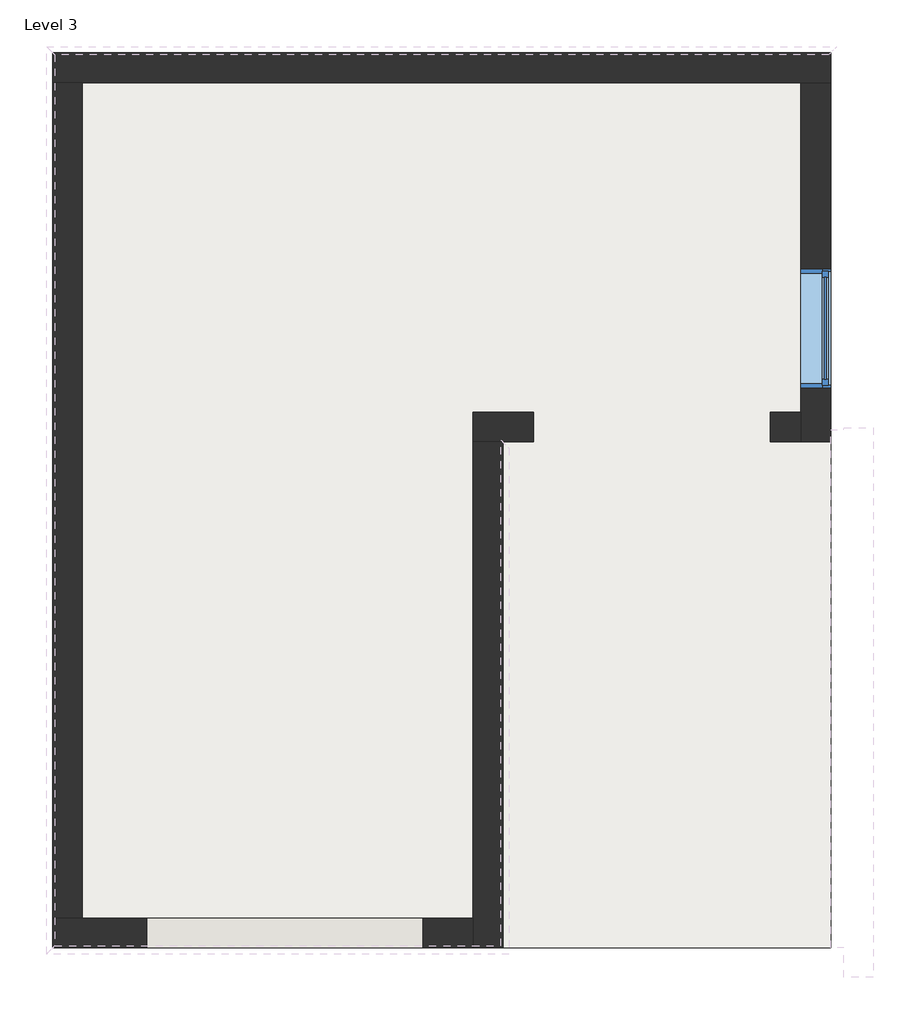
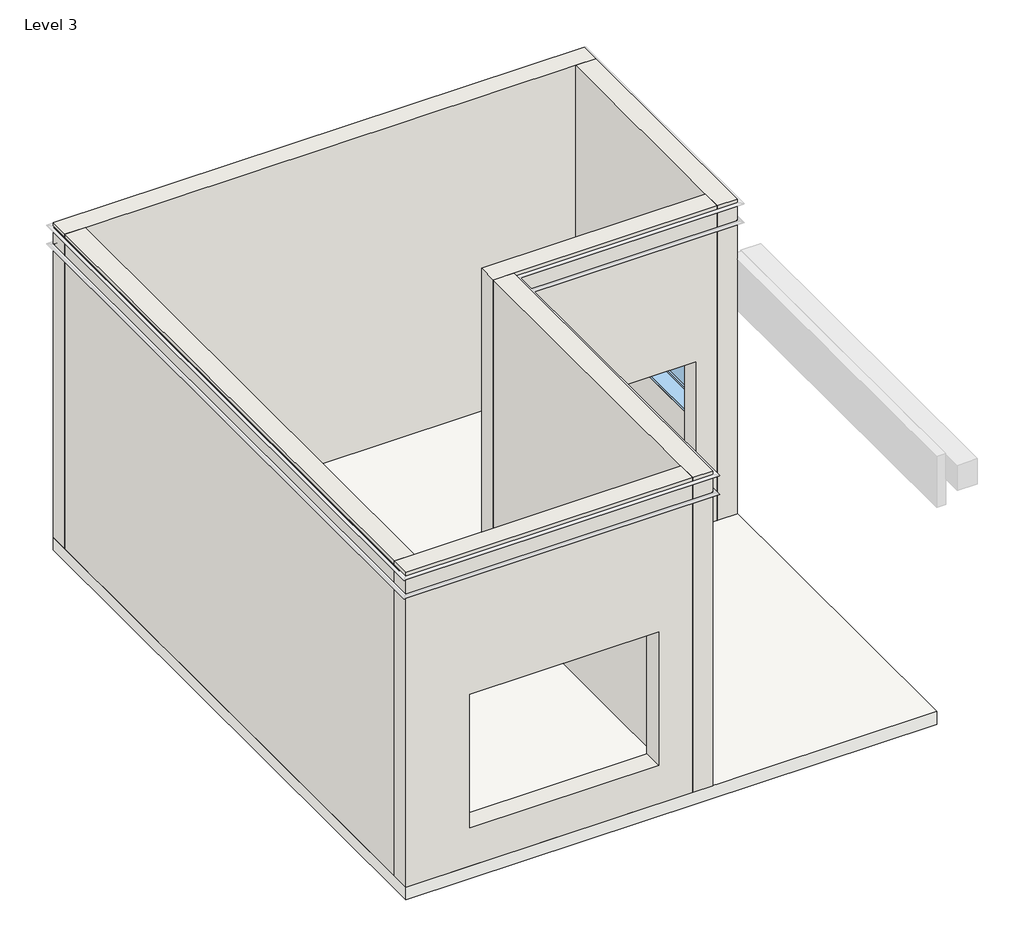
# One storey, part 1 of 2: 6 walls, 1 slab, 1 window.
"""IFC4 building model written with IfcOpenShell, lengths in millimetres."""

from ifc_helpers import new_model, si_unit, point, frame, frame_2d, origin, place, context, project, spatial, polyline, circle_curve, ellipse_curve, trimmed, segment, composite_curve, outline, extrude, faceted_brep, transform, mapped, element, save
from ifc_brep_helpers import plane_surface, cylinder_surface, advanced_brep
from components import window_c1f32544

model = new_model("IFC4")

# Units and contexts
model_context = context("Model", 3, world=origin())
ifc_project = project(units=[si_unit("LENGTHUNIT", "METRE", prefix="MILLI")], contexts=[model_context])

# Site, building, storey
site = spatial("IfcSite", under=ifc_project)
building = spatial("IfcBuilding", under=site)
storey = spatial("IfcBuildingStorey", under=building, Name="Level 3", Elevation=3200.4)

# Slab
placement = place(None, origin())
element("IfcSlab", 1, ObjectType="6\" floor", at=placement, inside=storey, context=model_context, shape_type="SweptSolid", body=[
    extrude(outline(polyline([(-7274.9953834, 7640.1262137), (-7274.9953834, 740.1262137), (-13274.9953834, 740.1262137), (-13274.9953834, 7640.1262137), (-7274.9953834, 7640.1262137)])), frame((0.0, 0.0, 3048.0), z_axis=(0.0, 0.0, 1.0), x_axis=(1.0, 0.0, 0.0)), (0.0, 0.0, 1.0), 152.4),
])

# Walls
element("IfcWall", 2, ObjectType="9\" wall", at=placement, inside=storey, context=model_context, shape_type="SolidModel", body=[
    faceted_brep([(-13274.9953834, 7411.5262137, 3200.4), (-13046.3953834, 7411.5262137, 3200.4), (-7503.5953834, 7411.5262137, 3200.4), (-7274.9953834, 7411.5262137, 3200.4), (-7274.9953834, 7411.5262137, 6692.9), (-7289.8797834, 7411.5262137, 6692.9), (-7289.8797834, 7411.5262137, 6921.5), (-7274.9953834, 7411.5262137, 6921.5), (-7274.9953834, 7411.5262137, 6962.2619583), (-7503.5953834, 7411.5262137, 6962.2619583), (-13046.3953834, 7411.5262137, 6962.2619583), (-13274.9953834, 7411.5262137, 6962.2619583), (-13274.9953834, 7411.5262137, 6921.5), (-13260.1109834, 7411.5262137, 6921.5), (-13260.1109834, 7411.5262137, 6692.9), (-13274.9953834, 7411.5262137, 6692.9), (-7274.9953834, 7640.1262137, 3200.4), (-13274.9953834, 7640.1262137, 3200.4), (-13274.9953834, 7640.1262137, 6692.9), (-7274.9953834, 7640.1262137, 6692.9), (-13274.9953834, 7640.1262137, 6962.2619583), (-7274.9953834, 7640.1262137, 6962.2619583), (-7274.9953834, 7640.1262137, 6921.5), (-13274.9953834, 7640.1262137, 6921.5), (-7289.8797834, 7625.2418137, 6921.5), (-13260.1109834, 7625.2418137, 6921.5), (-13260.1109834, 7625.2418137, 6692.9), (-7289.8797834, 7625.2418137, 6692.9)], [[[0, 1, 2, 3, 4, 5, 6, 7, 8, 9, 10, 11, 12, 13, 14, 15]], [[16, 17, 18, 19]], [[20, 21, 22, 23]], [[3, 2, 1, 0, 17, 16]], [[11, 10, 9, 8, 21, 20]], [[3, 16, 19, 4]], [[21, 8, 7, 22]], [[11, 20, 23, 12]], [[17, 0, 15, 18]], [[24, 25, 13, 12, 23, 22, 7, 6]], [[26, 27, 5, 4, 19, 18, 15, 14]], [[25, 26, 14, 13]], [[25, 24, 27, 26]], [[27, 24, 6, 5]]]),
    advanced_brep(
    [(-13274.9953834, 7411.5262137, 6907.55311), (-13274.9953834, 7411.5262137, 6706.84689), (-13267.3499834, 7411.5262137, 6716.943989), (-13267.3499834, 7411.5262137, 6897.456011), (-7274.9953834, 7411.5262137, 6706.84689), (-7274.9953834, 7411.5262137, 6907.55311), (-7282.6407834, 7411.5262137, 6897.456011), (-7282.6407834, 7411.5262137, 6716.943989), (-13274.9953834, 7640.1262137, 6706.84689), (-13274.9953834, 7640.1262137, 6907.55311), (-7274.9953834, 7640.1262137, 6907.55311), (-7274.9953834, 7640.1262137, 6706.84689), (-13267.3499834, 7632.4808137, 6897.456011), (-13267.3499834, 7632.4808137, 6716.943989), (-7282.6407834, 7632.4808137, 6897.456011), (-7282.6407834, 7632.4808137, 6716.943989)],
    [
        (0, 1),
        (1, 2, circle_curve(frame((-13277.8401834, 7411.5262137, 6716.943989), z_axis=(0.0, -1.0, 0.0), x_axis=(-1.0, 0.0, 0.0)), 10.4902)),
        (2, 3),
        (3, 0, circle_curve(frame((-13277.8401834, 7411.5262137, 6897.456011), z_axis=(0.0, -1.0, 0.0), x_axis=(-1.0, 0.0, 0.0)), 10.4902)),
        (4, 5),
        (5, 6, circle_curve(frame((-7272.1505834, 7411.5262137, 6897.456011), z_axis=(0.0, -1.0, 0.0), x_axis=(1.0, 0.0, 0.0)), 10.4902)),
        (6, 7),
        (7, 4, circle_curve(frame((-7272.1505834, 7411.5262137, 6716.943989), z_axis=(0.0, -1.0, 0.0), x_axis=(1.0, 0.0, 0.0)), 10.4902)),
        (8, 9),
        (9, 10),
        (10, 11),
        (11, 8),
        (4, 11),
        (10, 5),
        (0, 9),
        (8, 1),
        (12, 9, ellipse_curve(frame((-13277.8401834, 7642.9710137, 6897.456011), z_axis=(-0.7071067811865492, -0.7071067811865458, 0.0), x_axis=(-0.7071067811865457, 0.7071067811865492, 0.0)), 14.8353831, 10.4902)),
        (3, 12),
        (13, 12),
        (2, 13),
        (8, 13, ellipse_curve(frame((-13277.8401834, 7642.9710137, 6716.943989), z_axis=(-0.7071067811865492, -0.7071067811865458, 0.0), x_axis=(-0.7071067811865457, 0.7071067811865492, 0.0)), 14.8353831, 10.4902)),
        (12, 14),
        (14, 10, ellipse_curve(frame((-7272.1505834, 7642.9710137, 6897.456011), z_axis=(-0.7071067811865445, 0.7071067811865505, 0.0), x_axis=(0.7071067811865507, 0.7071067811865445, 0.0)), 14.8353831, 10.4902)),
        (13, 15),
        (15, 14),
        (11, 15, ellipse_curve(frame((-7272.1505834, 7642.9710137, 6716.943989), z_axis=(-0.7071067811865445, 0.7071067811865505, 0.0), x_axis=(0.7071067811865507, 0.7071067811865445, 0.0)), 14.8353831, 10.4902)),
        (14, 6),
        (15, 7),
    ],
    [
        plane_surface(frame((-13274.9953834, 7411.5262137, 3200.4), z_axis=(0.0, -1.0, 0.0), x_axis=(1.0, 0.0, 0.0))),
        plane_surface(frame((-13274.9953834, 7640.1262137, 3200.4), z_axis=(0.0, 1.0, 0.0), x_axis=(-1.0, 0.0, 0.0))),
        plane_surface(frame((-7274.9953834, 7640.1262137, 3200.4), z_axis=(1.0, 0.0, 0.0), x_axis=(0.0, 1.0, 0.0))),
        plane_surface(frame((-13274.9953834, 740.1262137, 3200.4), z_axis=(-1.0, 0.0, 0.0), x_axis=(0.0, -1.0, 0.0))),
        cylinder_surface(frame((-13277.8401834, 740.1262137, 6897.456011), z_axis=(0.0, 1.0, 0.0), x_axis=(-1.0, 0.0, 0.0)), 10.4902),
        plane_surface(frame((-13267.3499834, 740.1262137, 6897.456011), z_axis=(1.0, 0.0, 0.0), x_axis=(0.0, 1.0, 0.0))),
        cylinder_surface(frame((-13277.8401834, 740.1262137, 6716.943989), z_axis=(0.0, 1.0, 0.0), x_axis=(-1.0, 0.0, 0.0)), 10.4902),
        cylinder_surface(frame((-13274.9953834, 7642.9710137, 6897.456011), z_axis=(1.0, 0.0, 0.0), x_axis=(0.0, 1.0, 0.0)), 10.4902),
        plane_surface(frame((-13267.3499834, 7632.4808137, 6897.456011), z_axis=(0.0, -1.0, 0.0), x_axis=(1.0, 0.0, 0.0))),
        cylinder_surface(frame((-13274.9953834, 7642.9710137, 6716.943989), z_axis=(1.0, 0.0, 0.0), x_axis=(0.0, 1.0, 0.0)), 10.4902),
        cylinder_surface(frame((-7272.1505834, 7640.1262137, 6897.456011), z_axis=(0.0, -1.0, 0.0), x_axis=(1.0, 0.0, 0.0)), 10.4902),
        plane_surface(frame((-7282.6407834, 7632.4808137, 6897.456011), z_axis=(-1.0, 0.0, 0.0), x_axis=(0.0, -1.0, 0.0))),
        cylinder_surface(frame((-7272.1505834, 7640.1262137, 6716.943989), z_axis=(0.0, -1.0, 0.0), x_axis=(1.0, 0.0, 0.0)), 10.4902),
    ],
    [
        (0, [[1, 2, 3, 4]]),
        (0, [[5, 6, 7, 8]]),
        (1, [[9, 10, 11, 12]]),
        (2, [[-5, 13, -11, 14]]),
        (3, [[-1, 15, -9, 16]]),
        (4, [[17, -15, -4, 18]]),
        (5, [[19, -18, -3, 20]]),
        (6, [[21, -20, -2, -16]]),
        (7, [[22, 23, -10, -17]]),
        (8, [[-19, 24, 25, -22]]),
        (9, [[-24, -21, -12, 26]]),
        (10, [[-23, 27, -6, -14]]),
        (11, [[-25, 28, -7, -27]]),
        (12, [[-26, -13, -8, -28]]),
    ],
),
])
element("IfcWall", 3, ObjectType="9\" wall", at=placement, inside=storey, context=model_context, shape_type="SolidModel", body=[
    faceted_brep([(-7503.5953834, 7411.5262137, 3200.4), (-7503.5953834, 4868.7176199, 3200.4), (-7503.5953834, 4640.1176199, 3200.4), (-7503.5953834, 4640.1176199, 6692.9), (-7503.5953834, 4655.0020199, 6692.9), (-7503.5953834, 4655.0020199, 6921.5), (-7503.5953834, 4640.1176199, 6921.5), (-7503.5953834, 4640.1176199, 6962.2619583), (-7503.5953834, 4868.7176199, 6962.2619583), (-7503.5953834, 7411.5262137, 6962.2619583), (-7503.5953834, 5059.2176199, 5334.0), (-7503.5953834, 5059.2176199, 4114.8), (-7503.5953834, 5973.6176199, 4114.8), (-7503.5953834, 5973.6176199, 5334.0), (-7274.9953834, 4640.1176199, 3200.4), (-7274.9953834, 7411.5262137, 3200.4), (-7274.9953834, 7411.5262137, 6692.9), (-7274.9953834, 4640.1176199, 6692.9), (-7274.9953834, 5059.2176199, 4114.8), (-7274.9953834, 5059.2176199, 5334.0), (-7274.9953834, 5973.6176199, 5334.0), (-7274.9953834, 5973.6176199, 4114.8), (-7274.9953834, 7411.5262137, 6962.2619583), (-7274.9953834, 4640.1176199, 6962.2619583), (-7274.9953834, 4640.1176199, 6921.5), (-7274.9953834, 7411.5262137, 6921.5), (-7289.8797834, 7411.5262137, 6921.5), (-7289.8797834, 7411.5262137, 6692.9), (-7289.8797834, 4655.0020199, 6921.5), (-7289.8797834, 4655.0020199, 6692.9)], [[[0, 1, 2, 3, 4, 5, 6, 7, 8, 9], [10, 11, 12, 13]], [[14, 15, 16, 17], [18, 19, 20, 21]], [[22, 23, 24, 25]], [[2, 1, 0, 15, 14]], [[9, 8, 7, 23, 22]], [[0, 9, 22, 25, 26, 27, 16, 15]], [[11, 10, 19, 18]], [[12, 11, 18, 21]], [[13, 12, 21, 20]], [[10, 13, 20, 19]], [[2, 14, 17, 3]], [[23, 7, 6, 24]], [[5, 28, 26, 25, 24, 6]], [[27, 29, 4, 3, 17, 16]], [[28, 29, 27, 26]], [[29, 28, 5, 4]]]),
    advanced_brep(
    [(-7503.5953834, 4640.1176199, 6706.84689), (-7503.5953834, 4640.1176199, 6907.55311), (-7503.5953834, 4647.7630199, 6897.456011), (-7503.5953834, 4647.7630199, 6716.943989), (-7274.9953834, 7411.5262137, 6706.84689), (-7274.9953834, 7411.5262137, 6907.55311), (-7274.9953834, 4640.1176199, 6907.55311), (-7274.9953834, 4640.1176199, 6706.84689), (-7282.6407834, 7411.5262137, 6716.943989), (-7282.6407834, 7411.5262137, 6897.456011), (-7282.6407834, 4647.7630199, 6897.456011), (-7282.6407834, 4647.7630199, 6716.943989)],
    [
        (0, 1),
        (1, 2, circle_curve(frame((-7503.5953834, 4637.2728199, 6897.456011), z_axis=(-1.0, 0.0, 0.0), x_axis=(0.0, -1.0, 0.0)), 10.4902)),
        (2, 3),
        (3, 0, circle_curve(frame((-7503.5953834, 4637.2728199, 6716.943989), z_axis=(-1.0, 0.0, 0.0), x_axis=(0.0, -1.0, 0.0)), 10.4902)),
        (4, 5),
        (5, 6),
        (6, 7),
        (7, 4),
        (4, 8, circle_curve(frame((-7272.1505834, 7411.5262137, 6716.943989), z_axis=(0.0, 1.0, 0.0), x_axis=(1.0, 0.0, 0.0)), 10.4902)),
        (8, 9),
        (9, 5, circle_curve(frame((-7272.1505834, 7411.5262137, 6897.456011), z_axis=(0.0, 1.0, 0.0), x_axis=(1.0, 0.0, 0.0)), 10.4902)),
        (0, 7),
        (6, 1),
        (10, 6, ellipse_curve(frame((-7272.1505834, 4637.2728199, 6897.456011), z_axis=(0.7071067811865509, 0.707106781186544, 0.0), x_axis=(0.7071067811865439, -0.707106781186551, 0.0)), 14.8353831, 10.4902)),
        (9, 10),
        (11, 10),
        (8, 11),
        (7, 11, ellipse_curve(frame((-7272.1505834, 4637.2728199, 6716.943989), z_axis=(0.7071067811865509, 0.707106781186544, 0.0), x_axis=(0.7071067811865439, -0.707106781186551, 0.0)), 14.8353831, 10.4902)),
        (10, 2),
        (11, 3),
    ],
    [
        plane_surface(frame((-7503.5953834, 7640.1262137, 3200.4), z_axis=(-1.0, 0.0, 0.0), x_axis=(0.0, -1.0, 0.0))),
        plane_surface(frame((-7274.9953834, 7640.1262137, 3200.4), z_axis=(1.0, 0.0, 0.0), x_axis=(0.0, 1.0, 0.0))),
        plane_surface(frame((-13274.9953834, 7411.5262137, 3200.4), z_axis=(0.0, 1.0, 0.0), x_axis=(1.0, 0.0, 0.0))),
        plane_surface(frame((-11496.678825, 4640.1176199, 3200.4), z_axis=(0.0, -1.0, 0.0), x_axis=(1.0, 0.0, 0.0))),
        cylinder_surface(frame((-7272.1505834, 7640.1262137, 6897.456011), z_axis=(0.0, -1.0, 0.0), x_axis=(1.0, 0.0, 0.0)), 10.4902),
        plane_surface(frame((-7282.6407834, 7632.4808137, 6897.456011), z_axis=(-1.0, 0.0, 0.0), x_axis=(0.0, -1.0, 0.0))),
        cylinder_surface(frame((-7272.1505834, 7640.1262137, 6716.943989), z_axis=(0.0, -1.0, 0.0), x_axis=(1.0, 0.0, 0.0)), 10.4902),
        cylinder_surface(frame((-7274.9953834, 4637.2728199, 6897.456011), z_axis=(-1.0, 0.0, 0.0), x_axis=(0.0, -1.0, 0.0)), 10.4902),
        plane_surface(frame((-7282.6407834, 4647.7630199, 6897.456011), z_axis=(0.0, 1.0, 0.0), x_axis=(-1.0, 0.0, 0.0))),
        cylinder_surface(frame((-7274.9953834, 4637.2728199, 6716.943989), z_axis=(-1.0, 0.0, 0.0), x_axis=(0.0, -1.0, 0.0)), 10.4902),
    ],
    [
        (0, [[1, 2, 3, 4]]),
        (1, [[5, 6, 7, 8]]),
        (2, [[-5, 9, 10, 11]]),
        (3, [[-1, 12, -7, 13]]),
        (4, [[14, -6, -11, 15]]),
        (5, [[16, -15, -10, 17]]),
        (6, [[18, -17, -9, -8]]),
        (7, [[-14, 19, -2, -13]]),
        (8, [[-16, 20, -3, -19]]),
        (9, [[-18, -12, -4, -20]]),
    ],
),
])
element("IfcWall", 4, ObjectType="9\" wall", at=placement, inside=storey, context=model_context, shape_type="SweptSolid", body=[
    extrude(outline(polyline([(3200.4, -13046.3953834), (6962.2619583, -13046.3953834), (6962.2619583, -13274.9953834), (6921.5, -13274.9953834), (6921.5, -13260.1109834), (6692.9, -13260.1109834), (6692.9, -13274.9953834), (3200.4, -13274.9953834), (3200.4, -13046.3953834)])), frame((0.0, 968.7262137, 0.0), z_axis=(0.0, 1.0, 0.0), x_axis=(0.0, 0.0, 1.0)), (0.0, 0.0, 1.0), 6442.8),
    extrude(outline(composite_curve([segment(polyline([(6907.55311, -13274.9953834), (6706.84689, -13274.9953834)]), True, "CONTINUOUS"), segment(trimmed(circle_curve(frame_2d((6716.943989, -13277.8401834)), 10.4902), [point((6706.84689, -13274.9953834))], [point((6716.943989, -13267.3499834))], False, "CARTESIAN"), True, "CONTINUOUS"), segment(polyline([(6716.943989, -13267.3499834), (6897.456011, -13267.3499834)]), True, "CONTINUOUS"), segment(trimmed(circle_curve(frame_2d((6897.456011, -13277.8401834)), 10.4902), [point((6897.456011, -13267.3499834))], [point((6907.55311, -13274.9953834))], False, "CARTESIAN"), True, "CONTINUOUS")], self_intersect=False)), frame((0.0, 968.7262137, 0.0), z_axis=(0.0, 1.0, 0.0), x_axis=(0.0, 0.0, 1.0)), (0.0, 0.0, 1.0), 6442.8),
])
element("IfcWall", 5, ObjectType="9\" wall", at=placement, inside=storey, context=model_context, shape_type="SolidModel", body=[
    faceted_brep([(-10032.1297584, 4868.7176199, 6962.2619583), (-7503.5953834, 4868.7176199, 6962.2619583), (-7503.5953834, 4868.7176199, 3200.4), (-7739.1625709, 4868.7176199, 3200.4), (-7739.1625709, 4868.7176199, 5181.6), (-9567.9625709, 4868.7176199, 5181.6), (-9567.9625709, 4868.7176199, 3200.4), (-10032.1297584, 4868.7176199, 3200.4), (-7503.5953834, 4640.1176199, 6962.2619583), (-9803.5297584, 4640.1176199, 6962.2619583), (-10032.1297584, 4640.1176199, 6962.2619583), (-10032.1297584, 4640.1176199, 3200.4), (-9803.5297584, 4640.1176199, 3200.4), (-9567.9625709, 4640.1176199, 3200.4), (-9567.9625709, 4640.1176199, 5181.6), (-7739.1625709, 4640.1176199, 5181.6), (-7739.1625709, 4640.1176199, 3200.4), (-7503.5953834, 4640.1176199, 3200.4), (-7503.5953834, 4640.1176199, 6692.9), (-9803.5297584, 4640.1176199, 6692.9), (-9818.4141584, 4640.1176199, 6692.9), (-9818.4141584, 4640.1176199, 6921.5), (-9803.5297584, 4640.1176199, 6921.5), (-7503.5953834, 4640.1176199, 6921.5), (-7503.5953834, 4655.0020199, 6921.5), (-7503.5953834, 4655.0020199, 6692.9), (-9818.4141584, 4655.0020199, 6921.5), (-9818.4141584, 4655.0020199, 6692.9)], [[[0, 1, 2, 3, 4, 5, 6, 7]], [[8, 9, 10, 11, 12, 13, 14, 15, 16, 17, 18, 19, 20, 21, 22, 23]], [[11, 7, 6, 13, 12]], [[2, 17, 16, 3]], [[1, 0, 10, 9, 8]], [[0, 7, 11, 10]], [[2, 1, 8, 23, 24, 25, 18, 17]], [[5, 14, 13, 6]], [[15, 4, 3, 16]], [[14, 5, 4, 15]], [[21, 26, 24, 23, 22]], [[25, 27, 20, 19, 18]], [[26, 27, 25, 24]], [[27, 26, 21, 20]]]),
    advanced_brep(
    [(-7503.5953834, 4640.1176199, 6706.84689), (-7503.5953834, 4640.1176199, 6907.55311), (-9803.5297584, 4640.1176199, 6907.55311), (-9811.1751584, 4640.1176199, 6897.456011), (-9811.1751584, 4640.1176199, 6716.943989), (-9803.5297584, 4640.1176199, 6706.84689), (-7503.5953834, 4647.7630199, 6716.943989), (-7503.5953834, 4647.7630199, 6897.456011), (-9811.1751584, 4647.7630199, 6897.456011), (-9811.1751584, 4647.7630199, 6716.943989)],
    [
        (0, 1),
        (1, 2),
        (2, 3, circle_curve(frame((-9800.6849584, 4640.1176199, 6897.456011), z_axis=(0.0, -1.0, 0.0), x_axis=(1.0, 0.0, 0.0)), 10.4902)),
        (3, 4),
        (4, 5, circle_curve(frame((-9800.6849584, 4640.1176199, 6716.943989), z_axis=(0.0, -1.0, 0.0), x_axis=(1.0, 0.0, 0.0)), 10.4902)),
        (5, 0),
        (0, 6, circle_curve(frame((-7503.5953834, 4637.2728199, 6716.943989), z_axis=(1.0, 0.0, 0.0), x_axis=(0.0, -1.0, 0.0)), 10.4902)),
        (6, 7),
        (7, 1, circle_curve(frame((-7503.5953834, 4637.2728199, 6897.456011), z_axis=(1.0, 0.0, 0.0), x_axis=(0.0, -1.0, 0.0)), 10.4902)),
        (8, 2, ellipse_curve(frame((-9800.6849584, 4637.2728199, 6897.456011), z_axis=(0.7071067811865497, 0.7071067811865452, 0.0), x_axis=(-0.7071067811865456, 0.7071067811865496, 0.0)), 14.8353831, 10.4902)),
        (7, 8),
        (9, 8),
        (6, 9),
        (5, 9, ellipse_curve(frame((-9800.6849584, 4637.2728199, 6716.943989), z_axis=(0.7071067811865497, 0.7071067811865452, 0.0), x_axis=(-0.7071067811865456, 0.7071067811865496, 0.0)), 14.8353831, 10.4902)),
        (8, 3),
        (9, 4),
    ],
    [
        plane_surface(frame((-11496.678825, 4640.1176199, 3200.4), z_axis=(0.0, -1.0, 0.0), x_axis=(1.0, 0.0, 0.0))),
        plane_surface(frame((-7503.5953834, 7640.1262137, 3200.4), z_axis=(1.0, 0.0, 0.0), x_axis=(0.0, -1.0, 0.0))),
        cylinder_surface(frame((-7274.9953834, 4637.2728199, 6897.456011), z_axis=(-1.0, 0.0, 0.0), x_axis=(0.0, -1.0, 0.0)), 10.4902),
        plane_surface(frame((-7282.6407834, 4647.7630199, 6897.456011), z_axis=(0.0, 1.0, 0.0), x_axis=(-1.0, 0.0, 0.0))),
        cylinder_surface(frame((-7274.9953834, 4637.2728199, 6716.943989), z_axis=(-1.0, 0.0, 0.0), x_axis=(0.0, -1.0, 0.0)), 10.4902),
        cylinder_surface(frame((-9800.6849584, 4640.1176199, 6897.456011), z_axis=(0.0, -1.0, 0.0), x_axis=(1.0, 0.0, 0.0)), 10.4902),
        plane_surface(frame((-9811.1751584, 4647.7630199, 6897.456011), z_axis=(-1.0, 0.0, 0.0), x_axis=(0.0, -1.0, 0.0))),
        cylinder_surface(frame((-9800.6849584, 4640.1176199, 6716.943989), z_axis=(0.0, -1.0, 0.0), x_axis=(1.0, 0.0, 0.0)), 10.4902),
    ],
    [
        (0, [[1, 2, 3, 4, 5, 6]]),
        (1, [[-1, 7, 8, 9]]),
        (2, [[10, -2, -9, 11]]),
        (3, [[12, -11, -8, 13]]),
        (4, [[14, -13, -7, -6]]),
        (5, [[-10, 15, -3]]),
        (6, [[-12, 16, -4, -15]]),
        (7, [[-14, -5, -16]]),
    ],
),
])
element("IfcWall", 6, ObjectType="9\" wall", at=placement, inside=storey, context=model_context, shape_type="SolidModel", body=[
    faceted_brep([(-10032.1297584, 4640.1176199, 3200.4), (-10032.1297584, 968.7262137, 3200.4), (-10032.1297584, 740.1262137, 3200.4), (-10032.1297584, 740.1262137, 6692.9), (-10032.1297584, 755.0106137, 6692.9), (-10032.1297584, 755.0106137, 6921.5), (-10032.1297584, 740.1262137, 6921.5), (-10032.1297584, 740.1262137, 6962.2619583), (-10032.1297584, 968.7262137, 6962.2619583), (-10032.1297584, 4640.1176199, 6962.2619583), (-9803.5297584, 740.1262137, 3200.4), (-9803.5297584, 4640.1176199, 3200.4), (-9803.5297584, 4640.1176199, 6692.9), (-9803.5297584, 740.1262137, 6692.9), (-9803.5297584, 4640.1176199, 6962.2619583), (-9803.5297584, 740.1262137, 6962.2619583), (-9803.5297584, 740.1262137, 6921.5), (-9803.5297584, 4640.1176199, 6921.5), (-9818.4141584, 4640.1176199, 6921.5), (-9818.4141584, 4640.1176199, 6692.9), (-9818.4141584, 755.0106137, 6921.5), (-9818.4141584, 755.0106137, 6692.9)], [[[0, 1, 2, 3, 4, 5, 6, 7, 8, 9]], [[10, 11, 12, 13]], [[14, 15, 16, 17]], [[2, 1, 0, 11, 10]], [[9, 8, 7, 15, 14]], [[0, 9, 14, 17, 18, 19, 12, 11]], [[2, 10, 13, 3]], [[15, 7, 6, 16]], [[5, 20, 18, 17, 16, 6]], [[19, 21, 4, 3, 13, 12]], [[20, 21, 19, 18]], [[21, 20, 5, 4]]]),
    advanced_brep(
    [(-10032.1297584, 740.1262137, 6706.84689), (-10032.1297584, 740.1262137, 6907.55311), (-10032.1297584, 747.7716137, 6897.456011), (-10032.1297584, 747.7716137, 6716.943989), (-9803.5297584, 4640.1176199, 6706.84689), (-9803.5297584, 4640.1176199, 6907.55311), (-9803.5297584, 740.1262137, 6907.55311), (-9803.5297584, 740.1262137, 6706.84689), (-9811.1751584, 4640.1176199, 6716.943989), (-9811.1751584, 4640.1176199, 6897.456011), (-9811.1751584, 747.7716137, 6897.456011), (-9811.1751584, 747.7716137, 6716.943989)],
    [
        (0, 1),
        (1, 2, circle_curve(frame((-10032.1297584, 737.2814137, 6897.456011), z_axis=(-1.0, 0.0, 0.0), x_axis=(0.0, -1.0, 0.0)), 10.4902)),
        (2, 3),
        (3, 0, circle_curve(frame((-10032.1297584, 737.2814137, 6716.943989), z_axis=(-1.0, 0.0, 0.0), x_axis=(0.0, -1.0, 0.0)), 10.4902)),
        (4, 5),
        (5, 6),
        (6, 7),
        (7, 4),
        (4, 8, circle_curve(frame((-9800.6849584, 4640.1176199, 6716.943989), z_axis=(0.0, 1.0, 0.0), x_axis=(1.0, 0.0, 0.0)), 10.4902)),
        (8, 9),
        (9, 5, circle_curve(frame((-9800.6849584, 4640.1176199, 6897.456011), z_axis=(0.0, 1.0, 0.0), x_axis=(1.0, 0.0, 0.0)), 10.4902)),
        (0, 7),
        (6, 1),
        (10, 6, ellipse_curve(frame((-9800.6849584, 737.2814137, 6897.456011), z_axis=(0.7071067811865501, 0.7071067811865449, 0.0), x_axis=(0.7071067811865448, -0.7071067811865501, 0.0)), 14.8353831, 10.4902)),
        (9, 10),
        (11, 10),
        (8, 11),
        (7, 11, ellipse_curve(frame((-9800.6849584, 737.2814137, 6716.943989), z_axis=(0.7071067811865501, 0.7071067811865449, 0.0), x_axis=(0.7071067811865448, -0.7071067811865501, 0.0)), 14.8353831, 10.4902)),
        (10, 2),
        (11, 3),
    ],
    [
        plane_surface(frame((-10032.1297584, 4754.4176199, 3200.4), z_axis=(-1.0, 0.0, 0.0), x_axis=(0.0, -1.0, 0.0))),
        plane_surface(frame((-9803.5297584, 4754.4176199, 3200.4), z_axis=(1.0, 0.0, 0.0), x_axis=(0.0, 1.0, 0.0))),
        plane_surface(frame((-11496.678825, 4640.1176199, 3200.4), z_axis=(0.0, 1.0, 0.0), x_axis=(1.0, 0.0, 0.0))),
        plane_surface(frame((-7274.9953834, 740.1262137, 3200.4), z_axis=(0.0, -1.0, 0.0), x_axis=(1.0, 0.0, 0.0))),
        cylinder_surface(frame((-9800.6849584, 4640.1176199, 6897.456011), z_axis=(0.0, -1.0, 0.0), x_axis=(1.0, 0.0, 0.0)), 10.4902),
        plane_surface(frame((-9811.1751584, 4647.7630199, 6897.456011), z_axis=(-1.0, 0.0, 0.0), x_axis=(0.0, -1.0, 0.0))),
        cylinder_surface(frame((-9800.6849584, 4640.1176199, 6716.943989), z_axis=(0.0, -1.0, 0.0), x_axis=(1.0, 0.0, 0.0)), 10.4902),
        cylinder_surface(frame((-9803.5297584, 737.2814137, 6897.456011), z_axis=(-1.0, 0.0, 0.0), x_axis=(0.0, -1.0, 0.0)), 10.4902),
        plane_surface(frame((-9811.1751584, 747.7716137, 6897.456011), z_axis=(0.0, 1.0, 0.0), x_axis=(-1.0, 0.0, 0.0))),
        cylinder_surface(frame((-9803.5297584, 737.2814137, 6716.943989), z_axis=(-1.0, 0.0, 0.0), x_axis=(0.0, -1.0, 0.0)), 10.4902),
    ],
    [
        (0, [[1, 2, 3, 4]]),
        (1, [[5, 6, 7, 8]]),
        (2, [[-5, 9, 10, 11]]),
        (3, [[-1, 12, -7, 13]]),
        (4, [[14, -6, -11, 15]]),
        (5, [[16, -15, -10, 17]]),
        (6, [[18, -17, -9, -8]]),
        (7, [[-14, 19, -2, -13]]),
        (8, [[-16, 20, -3, -19]]),
        (9, [[-18, -12, -4, -20]]),
    ],
),
])
element("IfcWall", 7, ObjectType="9\" wall", at=placement, inside=storey, context=model_context, shape_type="SolidModel", body=[
    faceted_brep([(-10032.1297584, 968.7262137, 3200.4), (-13046.3953834, 968.7262137, 3200.4), (-13274.9953834, 968.7262137, 3200.4), (-13274.9953834, 968.7262137, 6692.9), (-13260.1109834, 968.7262137, 6692.9), (-13260.1109834, 968.7262137, 6921.5), (-13274.9953834, 968.7262137, 6921.5), (-13274.9953834, 968.7262137, 6962.2619583), (-13046.3953834, 968.7262137, 6962.2619583), (-10032.1297584, 968.7262137, 6962.2619583), (-12551.0953834, 968.7262137, 5252.1648635), (-12551.0953834, 968.7262137, 3657.6), (-10417.4953834, 968.7262137, 3657.6), (-10417.4953834, 968.7262137, 5252.1648635), (-13274.9953834, 740.1262137, 3200.4), (-10032.1297584, 740.1262137, 3200.4), (-10032.1297584, 740.1262137, 6692.9), (-13274.9953834, 740.1262137, 6692.9), (-12551.0953834, 740.1262137, 3657.6), (-12551.0953834, 740.1262137, 5252.1648635), (-10417.4953834, 740.1262137, 5252.1648635), (-10417.4953834, 740.1262137, 3657.6), (-10032.1297584, 740.1262137, 6962.2619583), (-13274.9953834, 740.1262137, 6962.2619583), (-13274.9953834, 740.1262137, 6921.5), (-10032.1297584, 740.1262137, 6921.5), (-10032.1297584, 755.0106137, 6921.5), (-10032.1297584, 755.0106137, 6692.9), (-13260.1109834, 755.0106137, 6921.5), (-13260.1109834, 755.0106137, 6692.9)], [[[0, 1, 2, 3, 4, 5, 6, 7, 8, 9], [10, 11, 12, 13]], [[14, 15, 16, 17], [18, 19, 20, 21]], [[22, 23, 24, 25]], [[2, 1, 0, 15, 14]], [[9, 8, 7, 23, 22]], [[2, 14, 17, 3]], [[23, 7, 6, 24]], [[0, 9, 22, 25, 26, 27, 16, 15]], [[11, 10, 19, 18]], [[13, 12, 21, 20]], [[13, 20, 19, 10]], [[11, 18, 21, 12]], [[5, 28, 26, 25, 24, 6]], [[27, 29, 4, 3, 17, 16]], [[28, 29, 27, 26]], [[29, 28, 5, 4]]]),
    advanced_brep(
    [(-13274.9953834, 968.7262137, 6706.84689), (-13274.9953834, 968.7262137, 6907.55311), (-13267.3499834, 968.7262137, 6897.456011), (-13267.3499834, 968.7262137, 6716.943989), (-10032.1297584, 740.1262137, 6706.84689), (-10032.1297584, 740.1262137, 6907.55311), (-13274.9953834, 740.1262137, 6907.55311), (-13274.9953834, 740.1262137, 6706.84689), (-10032.1297584, 747.7716137, 6716.943989), (-10032.1297584, 747.7716137, 6897.456011), (-13267.3499834, 747.7716137, 6897.456011), (-13267.3499834, 747.7716137, 6716.943989)],
    [
        (0, 1),
        (1, 2, circle_curve(frame((-13277.8401834, 968.7262137, 6897.456011), z_axis=(0.0, 1.0, 0.0), x_axis=(-1.0, 0.0, 0.0)), 10.4902)),
        (2, 3),
        (3, 0, circle_curve(frame((-13277.8401834, 968.7262137, 6716.943989), z_axis=(0.0, 1.0, 0.0), x_axis=(-1.0, 0.0, 0.0)), 10.4902)),
        (4, 5),
        (5, 6),
        (6, 7),
        (7, 4),
        (0, 7),
        (6, 1),
        (4, 8, circle_curve(frame((-10032.1297584, 737.2814137, 6716.943989), z_axis=(1.0, 0.0, 0.0), x_axis=(0.0, -1.0, 0.0)), 10.4902)),
        (8, 9),
        (9, 5, circle_curve(frame((-10032.1297584, 737.2814137, 6897.456011), z_axis=(1.0, 0.0, 0.0), x_axis=(0.0, -1.0, 0.0)), 10.4902)),
        (10, 6, ellipse_curve(frame((-13277.8401834, 737.2814137, 6897.456011), z_axis=(0.7071067811865452, -0.7071067811865499, 0.0), x_axis=(-0.7071067811865497, -0.7071067811865454, 0.0)), 14.8353831, 10.4902)),
        (9, 10),
        (11, 10),
        (8, 11),
        (7, 11, ellipse_curve(frame((-13277.8401834, 737.2814137, 6716.943989), z_axis=(0.7071067811865452, -0.7071067811865499, 0.0), x_axis=(-0.7071067811865497, -0.7071067811865454, 0.0)), 14.8353831, 10.4902)),
        (10, 2),
        (11, 3),
    ],
    [
        plane_surface(frame((-7274.9953834, 968.7262137, 3200.4), z_axis=(0.0, 1.0, 0.0), x_axis=(-1.0, 0.0, 0.0))),
        plane_surface(frame((-7274.9953834, 740.1262137, 3200.4), z_axis=(0.0, -1.0, 0.0), x_axis=(1.0, 0.0, 0.0))),
        plane_surface(frame((-13274.9953834, 740.1262137, 3200.4), z_axis=(-1.0, 0.0, 0.0), x_axis=(0.0, -1.0, 0.0))),
        plane_surface(frame((-10032.1297584, 4754.4176199, 3200.4), z_axis=(1.0, 0.0, 0.0), x_axis=(0.0, -1.0, 0.0))),
        cylinder_surface(frame((-9803.5297584, 737.2814137, 6897.456011), z_axis=(-1.0, 0.0, 0.0), x_axis=(0.0, -1.0, 0.0)), 10.4902),
        plane_surface(frame((-9811.1751584, 747.7716137, 6897.456011), z_axis=(0.0, 1.0, 0.0), x_axis=(-1.0, 0.0, 0.0))),
        cylinder_surface(frame((-9803.5297584, 737.2814137, 6716.943989), z_axis=(-1.0, 0.0, 0.0), x_axis=(0.0, -1.0, 0.0)), 10.4902),
        cylinder_surface(frame((-13277.8401834, 740.1262137, 6897.456011), z_axis=(0.0, 1.0, 0.0), x_axis=(-1.0, 0.0, 0.0)), 10.4902),
        plane_surface(frame((-13267.3499834, 747.7716137, 6897.456011), z_axis=(1.0, 0.0, 0.0), x_axis=(0.0, 1.0, 0.0))),
        cylinder_surface(frame((-13277.8401834, 740.1262137, 6716.943989), z_axis=(0.0, 1.0, 0.0), x_axis=(-1.0, 0.0, 0.0)), 10.4902),
    ],
    [
        (0, [[1, 2, 3, 4]]),
        (1, [[5, 6, 7, 8]]),
        (2, [[-1, 9, -7, 10]]),
        (3, [[-5, 11, 12, 13]]),
        (4, [[14, -6, -13, 15]]),
        (5, [[16, -15, -12, 17]]),
        (6, [[18, -17, -11, -8]]),
        (7, [[-14, 19, -2, -10]]),
        (8, [[-16, 20, -3, -19]]),
        (9, [[-18, -9, -4, -20]]),
    ],
),
])

# Window
window_shape = window_c1f32544(model_context)
element("IfcWindow", 8, ObjectType="Fixed : 36\" x 48\"", at=placement, inside=storey, context=model_context, shape_type="MappedRepresentation", body=[
    mapped(window_shape, transform((-7389.2953834, 5478.3176199, 3200.4), x_axis=(0.0, -1.0, 0.0), y_axis=(1.0, 0.0, 0.0), z_axis=(0.0, 0.0, 1.0))),
])

save(model, "model.ifc")

# Revit data of these elements
# Type "6\" floor"
#   Assembly Code = "B1010"
#   Function = 0
#   Layers, outside or top first: 0' - 6" no material (function 1)
# Type "9\" wall"
#   Assembly Code = "B2010"
#   Layers, outside or top first: 0' - 9" "Asphalt, Pavement, Light Grey" (function 1)
# Type "Fixed : 36\" x 48\""
#   Type Mark = "1"
#   Construction Type Id = "GSP4R"
#   Assembly Code = "B2020100"
#   Analytic Construction = "1/8 in Pilkington single glazing"
#   Visual Light Transmittance = 0.9
#   Solar Heat Gain Coefficient = 0.78
#   Heat Transfer Coefficient (U) = 0.6496 BTU/(h·ft²·°F)
#   Height = 4' - 0"
#   Default Sill Height = 3' - 0"
#   Width = 3' - 0"
#   Window Inset = 0' - 0 3/4"
#   Define Thermal Properties by = 1
#   Define Thermal Properties by = 1
#   Glass Pane Material = Glass
#   Sash Material = Sash
#   Wall Closure = (empty or 0)
# Element 1 (IfcSlab, "6\" floor")
#   Height Offset From Level = 0' - 0"
#   Phase Created = New Construction
#   Materials on its faces: "Default Floor"
# Elements 2, 3, 4, 5, 6, 7 (IfcWall, "9\" wall")
#   Top Offset = 12' - 4.1048"
#   Base Offset = 0' - 0"
#   wall height = 12' - 4.1048"
#   Phase Created = New Construction
#   Base Constraint = Level 3
#   Top Constraint = Level 3
#   Materials on its faces: "Asphalt, Pavement, Light Grey"
# Element 8 (IfcWindow, "Fixed : 36\" x 48\"")
#   Mark = "2"
#   Phase Created = New Construction
#   Materials on its faces: "Sash", "Glass"
# Materials
#   "Asphalt, Pavement, Light Grey": class "Generic", colour RGB 120 120 120, transparency 0, Description = "Asphalt or tarmac paving", Cost = 0
#   "Glass": class "Glass", colour RGB 0 128 192, transparency 0.75, Description = "Soda Lime Glass", Cost = 0
#   "Sash": class "Wood", colour RGB 224 178 126, transparency 0, Cost = 0
#   "Default Floor": colour RGB 128 128 128, transparency 0, Cost = 0
